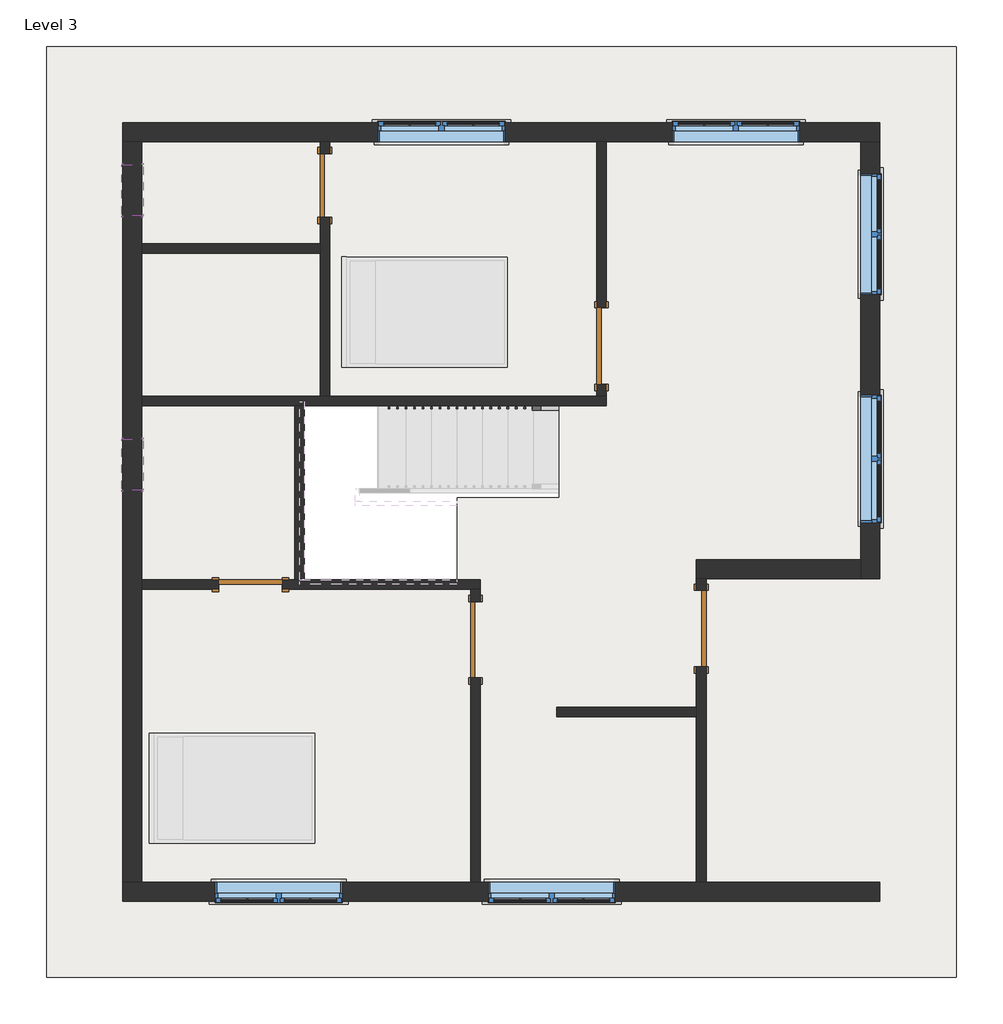
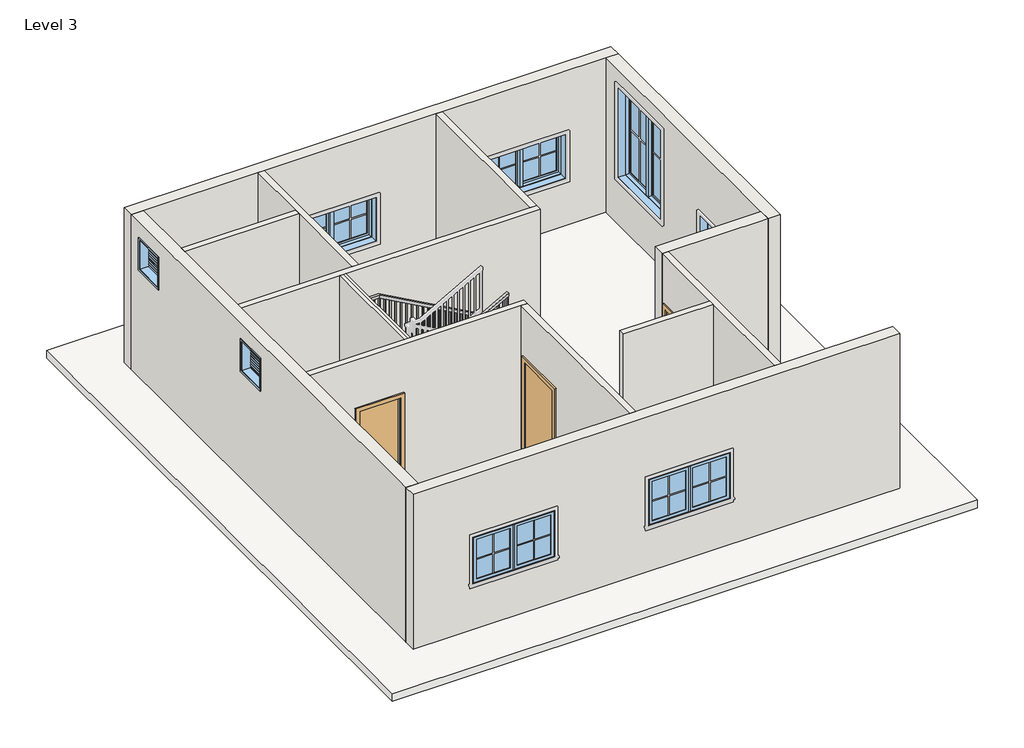
# One storey, part 1 of 2: 14 walls, 8 windows, 5 doors, 1 railing, 1 roof.
# Revit data of these elements (continued)
# Element 23 (IfcWindow, "Window-Casement-Double : WINDOW 6\"") (continued)
#   Interior Wall Closure = 0' - 2 1/4"
#   Frame Extension = 0' - 0 1/4"
#   Exterior Wall Closure = 0' - 1 1/4"
#   Interior Trim Visibility = yes
#   Exterior Trim Visibility = yes
#   Phase Created = New Construction
#   Materials on its faces: "Wood - Stained", "Glass", "Clad - White"
# Element 24 (IfcWindow, "Window-Casement-Double : WINDOW 6\"")
#   Mark = "18"
#   Window Inset = 0' - 0"
#   Interior Wall Closure = 0' - 2 1/4"
#   Frame Extension = 0' - 0 1/4"
#   Exterior Wall Closure = 0' - 1 1/4"
#   Interior Trim Visibility = yes
#   Exterior Trim Visibility = yes
#   Phase Created = New Construction
#   Materials on its faces: "Wood - Stained", "Glass", "Clad - White"
# Element 25 (IfcWindow, "Window-Casement-Double : WINDOW 6\"")
#   Mark = "19"
#   Window Inset = 0' - 0"
#   Interior Wall Closure = 0' - 2 1/4"
#   Frame Extension = 0' - 0 1/4"
#   Exterior Wall Closure = 0' - 1 1/4"
#   Interior Trim Visibility = yes
#   Exterior Trim Visibility = yes
#   Phase Created = New Construction
#   Materials on its faces: "Wood - Stained", "Glass", "Clad - White"
# Element 26 (IfcWindow, "Window-Casement-Double : WINDOW 6\"")
#   Mark = "20"
#   Window Inset = 0' - 0"
#   Interior Wall Closure = 0' - 2 1/4"
#   Frame Extension = 0' - 0 1/4"
#   Exterior Wall Closure = 0' - 1 1/4"
#   Interior Trim Visibility = yes
#   Exterior Trim Visibility = yes
#   Phase Created = New Construction
#   Materials on its faces: "Wood - Stained", "Glass", "Clad - White"
# Element 27 (IfcWindow, "Window-Casement-Double : WINDOW 6\"")
#   Mark = "21"
#   Window Inset = 0' - 0"
#   Interior Wall Closure = 0' - 2 1/4"
#   Frame Extension = 0' - 0 1/4"
#   Exterior Wall Closure = 0' - 1 1/4"
#   Interior Trim Visibility = yes
#   Exterior Trim Visibility = yes
#   Phase Created = New Construction
#   Materials on its faces: "Wood - Stained", "Glass", "Clad - White"
# Element 28 (IfcWindow, "Window-Louvers : 24\" x 24\"")
#   Mark = "22"
#   Blade Width = 1' - 10 1/2"
#   Phase Created = New Construction
#   Materials on its faces: "Birch"
# Element 29 (IfcWindow, "Window-Louvers : 24\" x 24\"")
#   Mark = "23"
#   Blade Width = 1' - 10 1/2"
#   Phase Created = New Construction
#   Materials on its faces: "Birch"
# Materials
#   "Door - Panel": class "Wood", colour RGB 210 159 95, transparency 0, Cost = 0
#   "Door - Frame": colour RGB 118 70 51, transparency 0, Cost = 0
#   "Wood - Stained": class "Wood", colour RGB 224 178 126, transparency 0, Cost = 0
#   "Glass": class "Glass", colour RGB 0 128 192, transparency 0.75, Description = "Soda Lime Glass", Cost = 0
#   "Clad - White": class "Wood", colour RGB 242 242 238, transparency 0, Cost = 0
#   "Birch": class "Wood", colour RGB 224 178 126, transparency 0, Description = "Betula Alleghaniensis", Cost = 0
#   "Default Wall": colour RGB 128 128 128, transparency 0, Cost = 0
